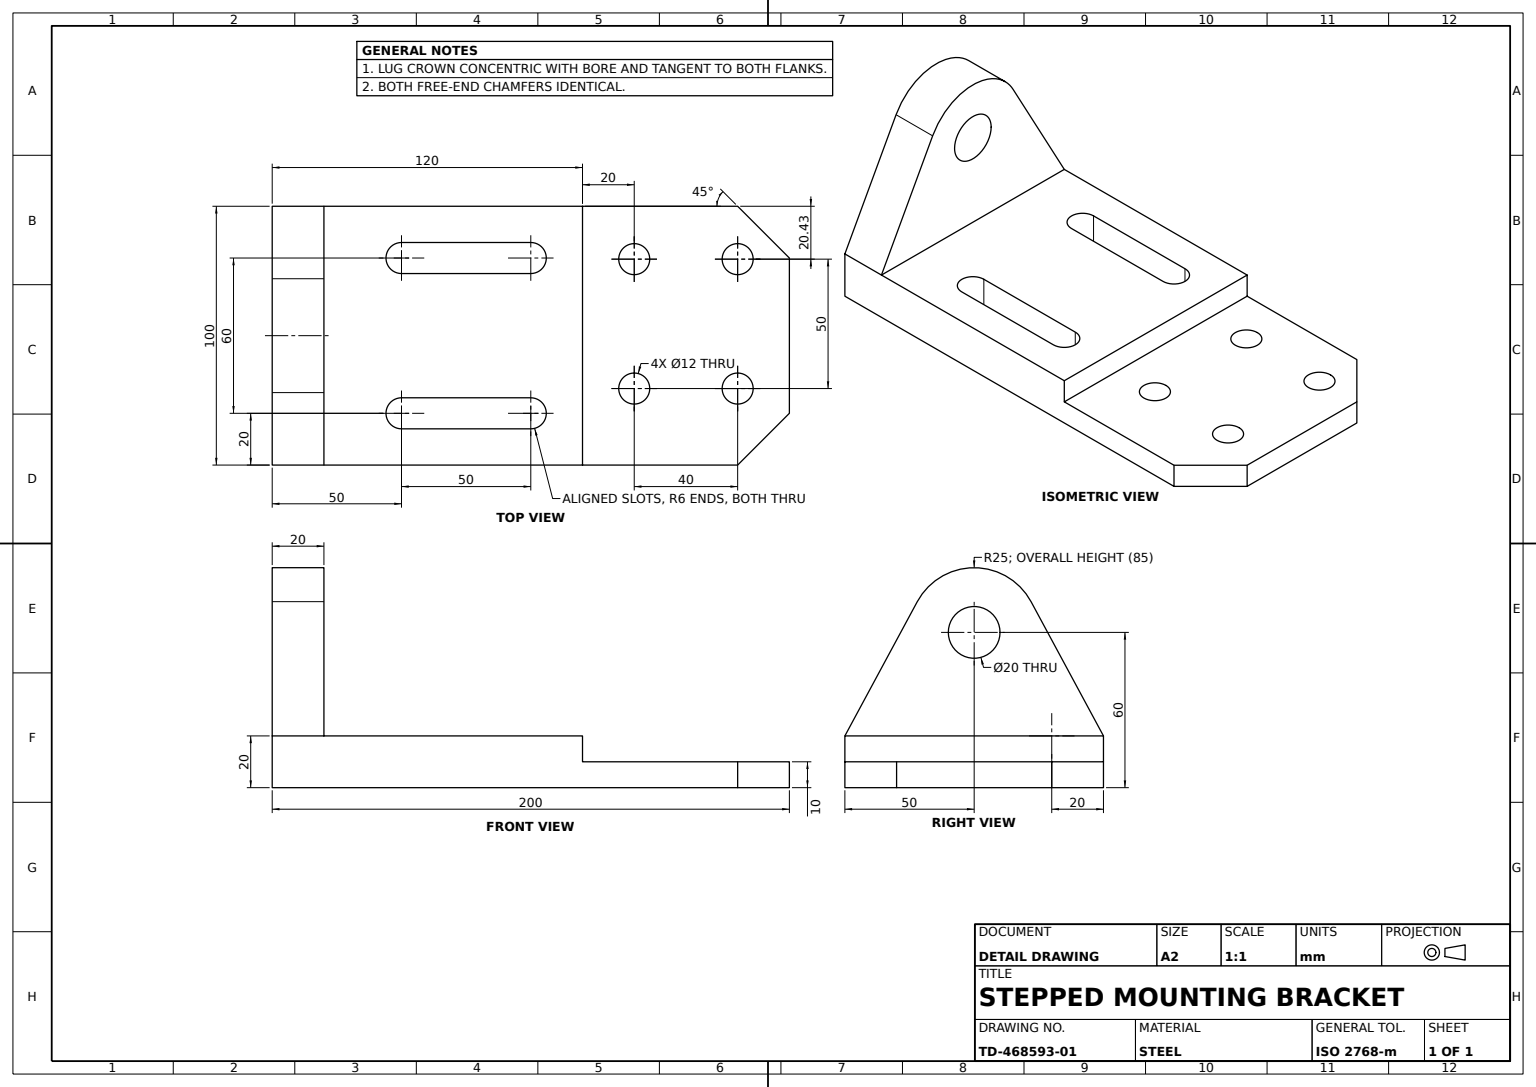
from build123d import *

# Parameters (mm, degrees)
BASE_PLATE_SKETCH_W       = 200
BASE_PLATE_SKETCH_H       = 100
BASE_PLATE_DEPTH          = 10
RAISED_PAD_SKETCH_W       = 120
RAISED_PAD_SKETCH_H       = 100
RAISED_PAD_DEPTH          = 10
CORNER_CHAMFER_A_SIZE     = 20
CORNER_CHAMFER_B_SIZE     = 20
ADJUSTMENT_SLOTS_2X_DEPTH = 20
LUG_SKETCH_R              = 10
PIERCED_LUG_DEPTH         = 20
MOUNTING_HOLES_SKETCH_R   = 6
MOUNTING_HOLES_4X_DEPTH   = 20


with BuildPart() as part:
    # Base Plate Sketch → Base Plate (new body)
    with BuildSketch(Plane(origin=(0, 0, 0), x_dir=(1, 0, 0), z_dir=(0, 1, 0))):
        Rectangle(BASE_PLATE_SKETCH_W, BASE_PLATE_SKETCH_H)
    extrude(amount=BASE_PLATE_DEPTH)

    # Raised Pad Sketch → Raised Pad (add)
    with BuildSketch(Plane(origin=(0, 10, 0), x_dir=(1, 0, 0), z_dir=(0, 1, 0))):
        with Locations((-40, 0)):
            Rectangle(RAISED_PAD_SKETCH_W, RAISED_PAD_SKETCH_H)
    extrude(amount=RAISED_PAD_DEPTH)

    # Corner Chamfer A
    corner_chamfer_a_edges = [part.edges().sort_by_distance(p)[0] for p in [
        (100, 5, 50),
    ]]
    chamfer(corner_chamfer_a_edges, length=CORNER_CHAMFER_A_SIZE)

    # Corner Chamfer B
    corner_chamfer_b_edges = [part.edges().sort_by_distance(p)[0] for p in [
        (100, 5, -50),
    ]]
    chamfer(corner_chamfer_b_edges, length=CORNER_CHAMFER_B_SIZE)

    # Adjustment Slots Sketch → Adjustment Slots 2x (cut)
    with BuildSketch(Plane(origin=(0, 20, 0), x_dir=(1, 0, 0), z_dir=(0, 1, 0))):
        with BuildLine():
            Line((-50, -24), (0, -24))
            ThreePointArc((0, -24), (6, -30), (0, -36))
            Line((0, -36), (-50, -36))
            ThreePointArc((-50, -36), (-56, -30), (-50, -24))
        make_face()
        with BuildLine():
            Line((-50, 24), (0, 24))
            ThreePointArc((0, 24), (6, 30), (0, 36))
            Line((0, 36), (-50, 36))
            ThreePointArc((-50, 36), (-56, 30), (-50, 24))
        make_face()
    extrude(amount=-ADJUSTMENT_SLOTS_2X_DEPTH, mode=Mode.SUBTRACT)

    # Lug Sketch → Pierced Lug (add)
    with BuildSketch(Plane.ZY.offset(100)):
        with BuildLine():
            Line((-21.999787954, 71.874734943), (-50, 20))
            Line((-50, 20), (50, 20))
            Line((50, 20), (21.999787954, 71.874734943))
            ThreePointArc((21.999787954, 71.874734943), (0, 85), (-21.999787954, 71.874734943))
        make_face()
        with Locations((0, 60)):
            Circle(LUG_SKETCH_R, mode=Mode.SUBTRACT)
    extrude(amount=-PIERCED_LUG_DEPTH)

    # Mounting Holes Sketch → Mounting Holes 4x (cut)
    with BuildSketch(Plane(origin=(0, 10, 0), x_dir=(1, 0, 0), z_dir=(0, 1, 0))):
        with Locations(Location((40, 29.565570893, 0), (0, 0, 270))):
            Circle(MOUNTING_HOLES_SKETCH_R)
        with Locations(Location((80, 29.565570893, 0), (0, 0, 270))):
            Circle(MOUNTING_HOLES_SKETCH_R)
        with Locations(Location((80, -20.434429107, 0), (0, 0, 90))):
            Circle(MOUNTING_HOLES_SKETCH_R)
        with Locations(Location((40, -20.434429107, 0), (0, 0, 90))):
            Circle(MOUNTING_HOLES_SKETCH_R)
    extrude(amount=-MOUNTING_HOLES_4X_DEPTH, mode=Mode.SUBTRACT)


solid = part.part
